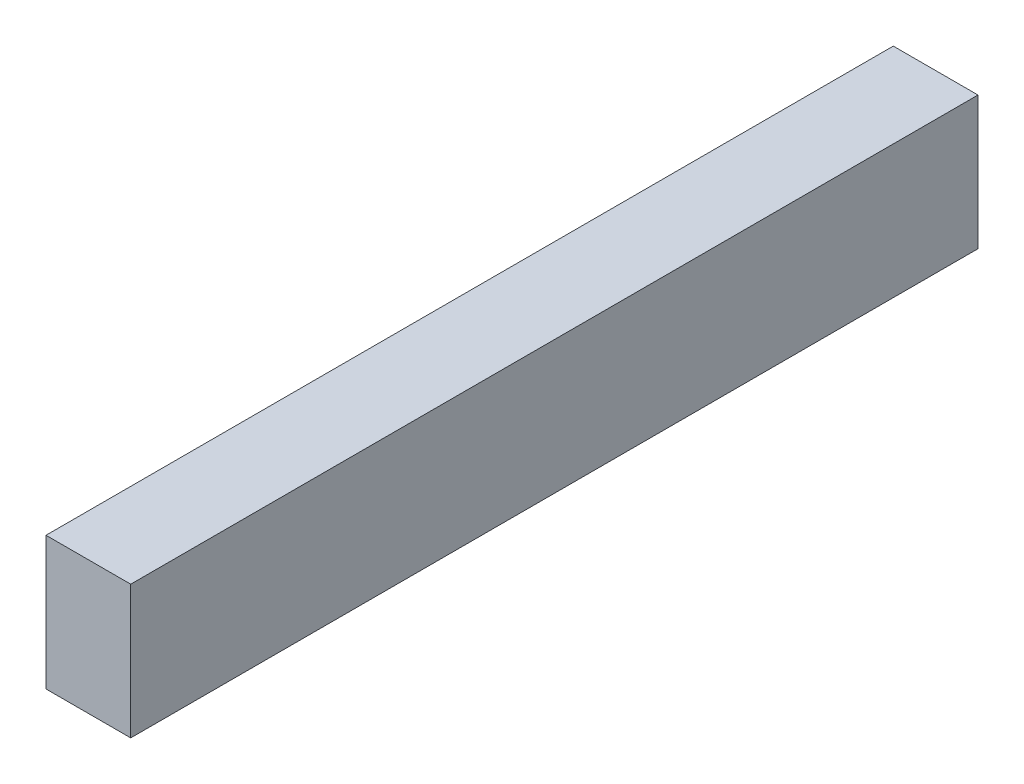
SolidWorks part; units mm, degrees
material "Plain Carbon Steel"
ref_plane "Front Plane" through (0, 0, 0) normal (0, 0, 1) x (1, 0, 0)
ref_plane "Top Plane" through (0, 0, 0) normal (0, 1, 0) x (1, 0, 0)
ref_plane "Right Plane" through (0, 0, 0) normal (1, 0, 0) x (0, 0, -1)
sketch "Key Section 22x14 Sketch" plane through (0, 0, 0) normal (0, 0, 1) x (1, 0, 0)
  line L1 (-7, -11) -> (7, -11)
  line L2 (-7, -11) -> (-7, 11)
  line L3 (-7, 11) -> (7, 11)
  line L4 (7, -11) -> (7, 11)
  line L5 (-7, -11) -> (7, 11) construction
  line L6 (-7, 11) -> (7, -11) construction
  point P0 (0, 0)
  dimension "D1" = 22
  dimension "D2" = 14
extrude "Key Body 140mm" add sketch "Key Section 22x14 Sketch" along normal mid plane 140
